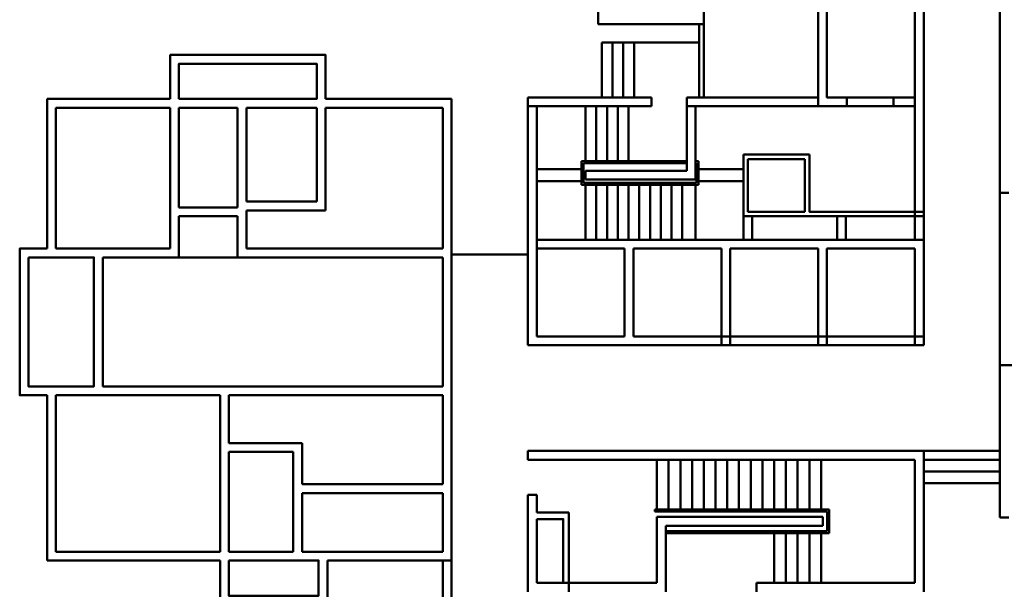
# Model space of a CAD drawing. Units: inches. Extents: x -105 to 1531, y -656 to 2003.
# Tile 2 of 6: x -28 to 979, y -29 to 553. Entities that reach past the tile are written whole.
import ezdxf

# ---------------------------------------------------------------- set-up
doc = ezdxf.new("R2010")
doc.units = ezdxf.units.IN
doc.header["$MEASUREMENT"] = 0
doc.layers.add('A-WALL', color=7, linetype='Continuous', lineweight=50)

msp = doc.modelspace()

# ---------------------------------------------------------------- linework, layer by layer
at = {"layer": 'A-WALL'}
for p, q in [((975, 743.6), (975, 220.1)), ((667.4, 473.6), (667.4, 548.6)), ((671.9, 548.6), (671.9, 473.6)), ((567.6, 473.6), (567.6, 529.8)), ((567.6, 529.8), (600.6, 529.8)), ((578.6, 473.6), (578.6, 529.8)), ((589.6, 473.6), (589.6, 529.8)), ((600.6, 473.6), (600.6, 529.8)), ((135, 508), (276, 508)), ((276, 508), (276, 472)), ((135, 487), (135, 499)), ((135, 472), (135, 487)), ((492, 319.1), (492, 473.6)), ((492, 473.6), (618.6, 473.6)), ((618.6, 473.6), (618.6, 464.6)), ((618.6, 464.6), (618.6, 473.6)), ((654.6, 464.6), (654.6, 473.6)), ((654.6, 473.6), (654.6, 464.6)), ((654.6, 473.6), (771, 473.6)), ((671.9, 473.6), (667.4, 473.6)), ((818.4, 473.6), (818.4, 464.6)), ((866.1, 464.6), (866.1, 473.6)), ((888, 464.6), (888, 473.6)), ((0, 472), (126, 472)), ((9, 472), (0, 472)), ((0, 472), (0, 360)), ((135, 472), (276, 472)), ((285, 472), (414, 472)), ((414, 169), (414, 472)), ((492, 464.6), (501, 464.6)), ((618.6, 464.6), (492, 464.6)), ((501, 464.6), (501, 323.6)), ((501, 464.6), (501, 328.1)), ((551, 408.3), (551, 464.6)), ((562, 408.3), (562, 464.6)), ((573, 408.3), (573, 464.6)), ((584, 408.3), (584, 464.6)), ((595, 408.3), (595, 464.6)), ((780, 464.6), (654.6, 464.6)), ((654.6, 398.5), (654.6, 464.6)), ((663.6, 389.5), (663.6, 464.6)), ((888, 464.6), (780, 464.6)), ((818.4, 464.6), (866.1, 464.6)), ((888, 356.6), (888, 464.6)), ((9, 463), (126, 463)), ((9, 319), (9, 463)), ((126, 319), (126, 463)), ((135, 463), (195, 463)), ((135, 361), (135, 463)), ((195, 361), (195, 463)), ((204, 367), (204, 463)), ((204, 463), (276, 463)), ((276, 367), (276, 463)), ((285, 358), (285, 463)), ((285, 463), (405, 463)), ((405, 319), (405, 463)), ((717, 415.1), (712.5, 415.1)), ((712.5, 415.1), (712.5, 356.6)), ((712.5, 356.6), (712.5, 415.1)), ((712.5, 328.1), (712.5, 415.1)), ((771, 415.1), (717, 415.1)), ((771, 415.1), (780, 415.1)), ((780, 415.1), (780, 356.6)), ((547, 408.3), (547, 384.3)), ((549, 408.3), (547, 408.3)), ((547, 408.3), (547, 384.3)), ((549, 408.3), (654.6, 408.3)), ((549, 406.3), (549, 386.3)), ((549, 406.3), (654.6, 406.3)), ((663.6, 408.3), (664.5, 408.3)), ((663.6, 406.3), (664.5, 406.3)), ((666.5, 408.3), (664.5, 408.3)), ((664.5, 386.3), (664.5, 406.3)), ((666.5, 384.3), (666.5, 408.3)), ((666.5, 384.3), (666.5, 408.3)), ((717, 356.6), (717, 410.6)), ((717, 410.6), (771, 410.6)), ((775.5, 410.6), (771, 410.6)), ((501, 400.1), (547, 400.1)), ((551, 398.5), (654.6, 398.5)), ((551, 389.5), (551, 398.5)), ((666.5, 400.1), (712.5, 400.1)), ((501, 388.1), (547, 388.1)), ((547, 384.3), (549, 384.3)), ((549, 386.3), (664.5, 386.3)), ((549, 386.3), (551, 386.3)), ((549, 384.3), (664.5, 384.3)), ((549, 384.3), (549, 384.3)), ((551, 389.5), (663.6, 389.5)), ((551, 384.3), (551, 328.1)), ((551, 328.1), (551, 384.3)), ((562, 328.1), (562, 384.3)), ((573, 328.1), (573, 384.3)), ((584, 328.1), (584, 384.3)), ((595, 328.1), (595, 384.3)), ((606, 328.1), (606, 384.3)), ((617, 328.1), (617, 384.3)), ((628, 328.1), (628, 384.3)), ((639, 328.1), (639, 384.3)), ((650, 328.1), (650, 384.3)), ((663.6, 328.1), (663.6, 384.3)), ((664.5, 384.3), (666.5, 384.3)), ((666.5, 388.1), (712.5, 388.1)), ((984, 376), (975, 376)), ((204, 367), (276, 367)), ((0, 319), (0, 360)), ((9, 319), (9, 360)), ((135, 361), (195, 361)), ((204, 358), (285, 358)), ((204, 319), (204, 358)), ((405, 319), (405, 360)), ((414, 0), (414, 360)), ((712.5, 356.6), (712.5, 328.1)), ((717, 356.6), (771, 356.6)), ((771, 356.6), (717, 356.6)), ((771, 356.6), (775.5, 356.6)), ((780, 356.6), (897, 356.6)), ((888, 356.6), (888, 328.1)), ((135, 352), (195, 352)), ((135, 310), (135, 352)), ((195, 310), (195, 352)), ((712.5, 352.1), (897, 352.1)), ((721.5, 328.1), (721.5, 352.1)), ((808.4, 328.1), (808.4, 352.1)), ((817.4, 328.1), (817.4, 352.1)), ((897, 328.1), (897, 352.1)), ((501, 319.1), (501, 328.1)), ((501, 328.1), (897, 328.1)), ((712.5, 328.1), (721.5, 328.1)), ((888, 328.1), (897, 328.1)), ((897, 328.1), (897, 319.1)), ((9, 319), (126, 319)), ((204, 319), (405, 319)), ((414, 313.1), (492, 313.1)), ((492, 319.1), (492, 229.1)), ((501, 229.1), (501, 319.1)), ((501, 319.1), (591, 319.1)), ((513, 319.1), (591, 319.1)), ((591, 319.1), (591, 229.1)), ((591, 319.1), (591, 229.1)), ((600, 229.1), (600, 319.1)), ((600, 319.1), (690, 319.1)), ((612, 319.1), (690, 319.1)), ((690, 319.1), (690, 229.1)), ((690, 319.1), (690, 229.1)), ((699, 229.1), (699, 319.1)), ((699, 319.1), (789, 319.1)), ((711, 319.1), (789, 319.1)), ((789, 319.1), (789, 229.1)), ((789, 319.1), (789, 229.1)), ((798, 229.1), (798, 319.1)), ((798, 319.1), (888, 319.1)), ((810, 319.1), (888, 319.1)), ((888, 319.1), (888, 229.1)), ((888, 319.1), (888, 229.1)), ((897, 229.1), (897, 319.1)), ((-19, 178), (-19, 310)), ((-19, 310), (0, 310)), ((0, 310), (48, 310)), ((48, 178), (48, 310)), ((57, 178), (57, 310)), ((57, 310), (405, 310)), ((405, 178), (405, 310)), ((405, 178), (405, 310)), ((492, 220.1), (492, 229.1)), ((591, 229.1), (501, 229.1)), ((501, 229.1), (591, 229.1)), ((690, 229.1), (600, 229.1)), ((600, 229.1), (897, 229.1)), ((690, 229.1), (699, 229.1)), ((690, 220.1), (690, 229.1)), ((789, 229.1), (699, 229.1)), ((699, 220.1), (699, 229.1)), ((789, 229.1), (798, 229.1)), ((789, 220.1), (789, 229.1)), ((888, 229.1), (798, 229.1)), ((798, 220.1), (798, 229.1)), ((888, 229.1), (897, 229.1)), ((888, 220.1), (888, 229.1)), ((897, 220.1), (897, 229.1)), ((492, 220.1), (897, 220.1)), ((975, 220.1), (975, 112.1)), ((1169, 199.9), (975, 199.9)), ((48, 178), (-19, 178)), ((0, 178), (48, 178)), ((57, 178), (405, 178)), ((0, 0), (0, 169)), ((9, 9), (9, 169)), ((9, 169), (177, 169)), ((177, 9), (177, 169)), ((186, 120), (186, 169)), ((186, 169), (405, 169)), ((405, 78), (405, 169)), ((186, 120), (261, 120)), ((186, 9), (186, 111)), ((186, 111), (252, 111)), ((252, 9), (252, 111)), ((261, 78), (261, 120)), ((492, 112.1), (560, 112.1)), ((897, 112.1), (492, 112.1)), ((492, 103.1), (492, 112.1)), ((975, 112.1), (560, 112.1)), ((897, 103.1), (897, 112.1)), ((897, -31.9), (897, 112.1)), ((975, 112.1), (975, 43.9)), ((888, 103.1), (492, 103.1)), ((888, 103.1), (560, 103.1)), ((623.8, 103.1), (623.8, 103.1)), ((624, 52.1), (624, 103.1)), ((636, 52.1), (636, 103.1)), ((648, 52.1), (648, 103.1)), ((660, 52.1), (660, 103.1)), ((672, 52.1), (672, 103.1)), ((684, 52.1), (684, 103.1)), ((696, 52.1), (696, 103.1)), ((708, 52.1), (708, 103.1)), ((720, 52.1), (720, 103.1)), ((732, 52.1), (732, 103.1)), ((744, 52.1), (744, 103.1)), ((756, 52.1), (756, 103.1)), ((768, 52.1), (768, 103.1)), ((780, 52.1), (780, 103.1)), ((792, 52.1), (792, 103.1)), ((888, 103.1), (798.2, 103.1)), ((888, -22.9), (888, 103.1)), ((975, 103.1), (897, 103.1)), ((975, 91.1), (897, 91.1)), ((261, 78), (405, 78)), ((975, 79.1), (897, 79.1)), ((261, 9), (261, 69)), ((261, 69), (405, 69)), ((405, 9), (405, 69)), ((492, -31.9), (492, 67.1)), ((492, 67.1), (501, 67.1)), ((501, 67.1), (501, 49.1)), ((501, 49.1), (501, 67.1)), ((621.8, 52.1), (800.2, 52.1)), ((621.8, 50.1), (621.8, 52.1)), ((800.2, 52.1), (800.2, 28.1)), ((534, 49.1), (501, 49.1)), ((501, -22.9), (501, 42.4)), ((534, -31.9), (534, 49.1)), ((623.8, 50.1), (621.8, 50.1)), ((623.8, 50.1), (798.2, 50.1)), ((624, 44.6), (793.7, 44.6)), ((624, -22.9), (624, 44.6)), ((793.7, 44.6), (793.7, 35.6)), ((798.2, 50.1), (798.2, 30.1)), ((975, 43.9), (984, 43.9)), ((633, -31.9), (633, 35.6)), ((633, 35.6), (793.7, 35.6)), ((633, 30.1), (798.2, 30.1)), ((633, 28.1), (800.2, 28.1)), ((744, -22.9), (744, 28.1)), ((756, -22.9), (756, 28.1)), ((768, -22.9), (768, 28.1)), ((780, -22.9), (780, 28.1)), ((792, -22.9), (792, 28.1)), ((0, 0), (177, 0)), ((9, 9), (177, 9)), ((186, 9), (252, 9)), ((186, 9), (252, 9)), ((186, 0), (277.8, 0)), ((186, 0), (186, -27)), ((186, 0), (277.8, 0)), ((261, 9), (405, 9)), ((261, 9), (360, 9)), ((277.8, -36), (277.8, 0)), ((286.8, 0), (414, 0)), ((286.8, 0), (360, 0)), ((405, -69), (405, 0)), ((405, 0), (414, 0)), ((414, 0), (414, -78)), ((624, -22.9), (501, -22.9)), ((525, -22.9), (624, -22.9)), ((888, -22.9), (725.8, -22.9)), ((725.8, -22.9), (725.8, -31.9))]:
    msp.add_line(p, q, dxfattribs=at)
for points in [[(888, 464.6), (789, 464.6), (789, 602.6), (849, 602.6)], [(897, 602.6), (897, 464.6)], [(564, 593.6), (564, 548.6), (671.9, 548.6), (671.9, 593.6)], [(587.3, 548.6), (576.5, 548.6)], [(608.7, 548.6), (597.9, 548.6)], [(619.5, 548.6), (608.7, 548.6)], [(630.3, 548.6), (619.5, 548.6)], [(641.1, 548.6), (630.3, 548.6)], [(651.9, 548.6), (641.1, 548.6)], [(595, 529.8), (667.4, 529.8)], [(285, 472), (285, 517), (126, 517), (126, 472)], [(618.6, 473.6), (595, 473.6)], [(789, 473.6), (771, 473.6)], [(888, 473.6), (798, 473.6)], [(897, 352.1), (897, 473.6)], [(654.6, 464.6), (654.6, 464.6), (654.6, 408.3), (595, 408.3), (595, 464.6), (618.6, 464.6)], [(780, 415.1), (780, 356.6), (888, 356.6), (888, 464.6), (780, 464.6)], [(135, 463), (195, 463)], [(204, 463), (276, 463)], [(775.5, 410.6), (775.5, 356.6)], [(0, 169), (-28, 169), (-28, 319), (0, 319)], [(9, 319), (57, 319)], [(57, 310), (57, 178)], [(57, 169), (9, 169)], [(501, 42.4), (528.2, 42.4), (528.2, 11.9)], [(528.2, 12.6), (528.2, -22.9)], [(286.8, 0), (286.8, -45), (177, -45), (177, 0)], [(186, 9), (252, 9)], [(261, 9), (286.8, 9)]]:
    msp.add_lwpolyline(points, dxfattribs=at)
for points in [[(888, 473.6), (798, 473.6), (798, 593.6), (888, 593.6)], [(135, 472), (276, 472), (276, 508), (135, 508)], [(654.6, 473.6), (654.6, 473.6)], [(-19, 310), (48, 310), (48, 178), (-19, 178)], [(186, 0), (277.8, 0), (277.8, -36), (186, -36)]]:
    msp.add_lwpolyline(points, close=True, dxfattribs=at)

doc.saveas('drawing.dxf')
